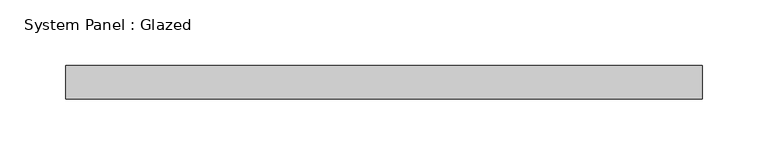
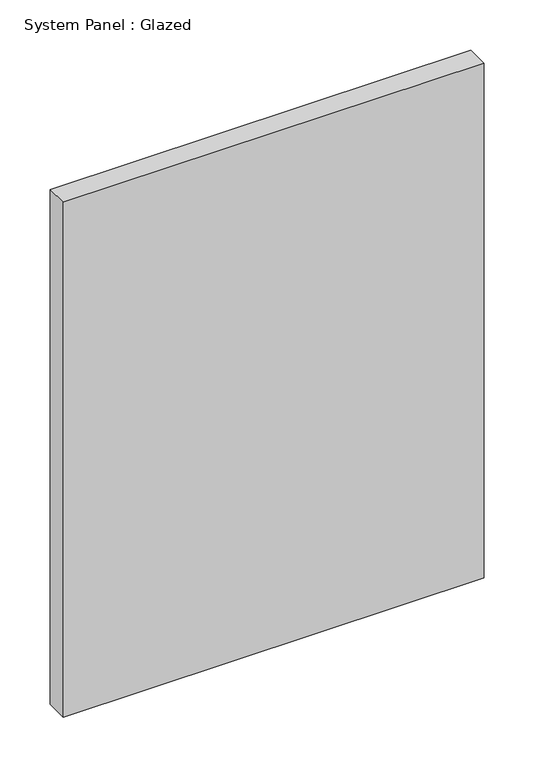
"""IFC4 building model written with IfcOpenShell, lengths in millimetres: plate geometry, System Panel : Glazed."""

from ifc_helpers import new_model, si_unit, origin, origin_with_axes, place, context, project, spatial, polyline, outline, extrude, source, transform, mapped, element, save


def system_panel_glazed_a0fb9759(model_context):
    return source(origin(), model_context, "Body", "SweptSolid", [
        extrude(outline(polyline([(241.3, 19.05), (-241.3, 19.05), (-241.3, 44.45), (241.3, 44.45), (241.3, 19.05)])), origin_with_axes(), (0.0, 0.0, 1.0), 624.5585391),
    ])


if __name__ == "__main__":
    model = new_model("IFC4")
    model_context = context("Model", 3, world=origin())
    ifc_project = project(units=[si_unit("LENGTHUNIT", "METRE", prefix="MILLI")], contexts=[model_context])
    site = spatial("IfcSite", under=ifc_project)
    building = spatial("IfcBuilding", under=site)
    placement = place(None, origin())
    system_panel_glazed_shape = system_panel_glazed_a0fb9759(model_context)
    element("IfcPlate", 1, ObjectType="System Panel : Glazed", at=placement, inside=building, context=model_context, shape_type="MappedRepresentation", body=[
        mapped(system_panel_glazed_shape, transform((0.0, 0.0, 0.0), x_axis=(1.0, 0.0, 0.0), y_axis=(0.0, 1.0, 0.0), z_axis=(0.0, 0.0, 1.0))),
    ])
    save(model, "model.ifc")

# Revit data of these elements
# Type "System Panel : Glazed"
#   Construction Type Id = "GSP4R"
#   Analytic Construction = "1/8 in Pilkington single glazing"
#   Visual Light Transmittance = 0.9
#   Solar Heat Gain Coefficient = 0.86
#   Heat Transfer Coefficient (U) = 1.18115 BTU/(h·ft²·°F)
#   Define Thermal Properties by = 1
# Element 1 (IfcPlate, "System Panel : Glazed")
#   Materials on its faces: "Glass"
# Materials
#   "Glass": class "Glass", colour RGB 0 128 192, transparency 0.75, Description = "Soda Lime Glass", Cost = 0
